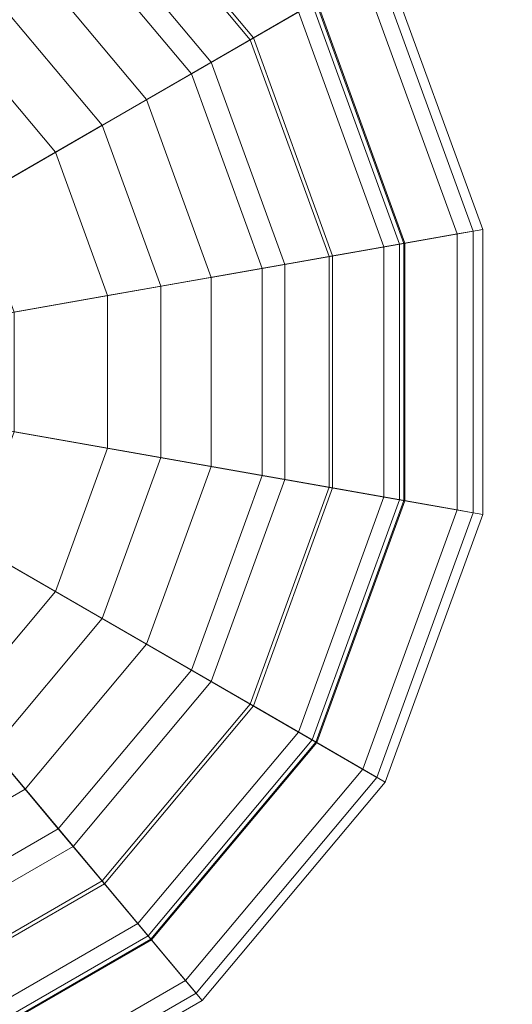
# Model space of a CAD drawing. Units: inches. Extents: x 375 to 1122, y 27 to 1069.
# Tile 130 of 155: x 722.65 to 723.463, y 901.45 to 903.075. Entities that reach past the tile are written whole.
import ezdxf

# ---------------------------------------------------------------- set-up
doc = ezdxf.new("R2010")
doc.units = ezdxf.units.IN
doc.layers.add('A-ANNO-DIMS', color=2, linetype='Continuous', lineweight=18)
doc.layers.add('Furniture', color=30, linetype='Continuous', lineweight=18)
doc.styles.get("Standard").update_dxf_attribs({"font": 'arial.ttf'})
doc.dimstyles.new('ISO-25', dxfattribs={"dimtxt": 12, "dimasz": 2.5, "dimexe": 1.5, "dimexo": 1.5, "dimtad": 1, "dimdec": 1, "dimlunit": 3, "dimtxsty": 'Standard', "dimblk": 'ARCHTICK', "dimcen": 2.5, "dimadec": 0, "dimazin": 0, "dimtfac": 1, "dimtdec": 1, "dimtmove": 0, "dimatfit": 3, "dimfxl": 1.5, "dimfxlon": 1, "dimarcsym": 0})

# ---------------------------------------------------------------- blocks, each defined once
blk = doc.blocks.new('A$C403C54AD')
for points in [[(0.890422, 0.958466, -0.039553), (0.889855, 0.961682, -0.042784), (0.878804, 0.95766, -0.042784), (0.880436, 0.954832, -0.039553)], [(0.889855, 0.961682, -0.042784), (0.895735, 0.928335, -0.039705), (0.895735, 0.928335, -0.039705), (0.878804, 0.95766, -0.042784)], [(0.901048, 0.958466, -0.039553), (0.901615, 0.961682, -0.042784), (0.889855, 0.961682, -0.042784), (0.890422, 0.958466, -0.039553)], [(0.901615, 0.961682, -0.042784), (0.895735, 0.928335, -0.039705), (0.895735, 0.928335, -0.039705), (0.889855, 0.961682, -0.042784)], [(0.912666, 0.95766, -0.042784), (0.895735, 0.928335, -0.039705), (0.895735, 0.928335, -0.039705), (0.901615, 0.961682, -0.042784)], [(0.911033, 0.954832, -0.039553), (0.912666, 0.95766, -0.042784), (0.901615, 0.961682, -0.042784), (0.901048, 0.958466, -0.039553)], [(0.890429, 0.958426, 0.1202), (0.889924, 0.961289, 0.106976), (0.879003, 0.957315, 0.106976), (0.880457, 0.954797, 0.1202)], [(0.889924, 0.961289, 0.106976), (0.890041, 0.960625, 0.078734), (0.87934, 0.95673, 0.078734), (0.879003, 0.957315, 0.106976)], [(0.901041, 0.958426, 0.1202), (0.901545, 0.961289, 0.106976), (0.889924, 0.961289, 0.106976), (0.890429, 0.958426, 0.1202)], [(0.901545, 0.961289, 0.106976), (0.901428, 0.960625, 0.078734), (0.890041, 0.960625, 0.078734), (0.889924, 0.961289, 0.106976)], [(0.911013, 0.954797, 0.1202), (0.912466, 0.957315, 0.106976), (0.901545, 0.961289, 0.106976), (0.901041, 0.958426, 0.1202)], [(0.912466, 0.957315, 0.106976), (0.912129, 0.95673, 0.078734), (0.901428, 0.960625, 0.078734), (0.901545, 0.961289, 0.106976)], [(0.890041, 0.960625, 0.078734), (0.890973, 0.955342, 0.060725), (0.882023, 0.952084, 0.060725), (0.87934, 0.95673, 0.078734)], [(0.901428, 0.960625, 0.078734), (0.900497, 0.955342, 0.060725), (0.890973, 0.955342, 0.060725), (0.890041, 0.960625, 0.078734)], [(0.912129, 0.95673, 0.078734), (0.909447, 0.952084, 0.060725), (0.900497, 0.955342, 0.060725), (0.901428, 0.960625, 0.078734)], [(0.893266, 0.942333, -0.036278), (0.890422, 0.958466, -0.039553), (0.880436, 0.954832, -0.039553), (0.888627, 0.940645, -0.036278)], [(0.891296, 0.953506, 0.129606), (0.890429, 0.958426, 0.1202), (0.880457, 0.954797, 0.1202), (0.882955, 0.95047, 0.129606)], [(0.890459, 0.958252, 0.106759), (0.890947, 0.955485, 0.119395), (0.88195, 0.95221, 0.119395), (0.880545, 0.954643, 0.106759)], [(0.890574, 0.957604, 0.079219), (0.890459, 0.958252, 0.106759), (0.880545, 0.954643, 0.106759), (0.880874, 0.954073, 0.079219)], [(0.898203, 0.942333, -0.036278), (0.901048, 0.958466, -0.039553), (0.890422, 0.958466, -0.039553), (0.893266, 0.942333, -0.036278)], [(0.900173, 0.953506, 0.129606), (0.901041, 0.958426, 0.1202), (0.890429, 0.958426, 0.1202), (0.891296, 0.953506, 0.129606)], [(0.90101, 0.958252, 0.106759), (0.900522, 0.955485, 0.119395), (0.890947, 0.955485, 0.119395), (0.890459, 0.958252, 0.106759)], [(0.900896, 0.957604, 0.079219), (0.90101, 0.958252, 0.106759), (0.890459, 0.958252, 0.106759), (0.890574, 0.957604, 0.079219)], [(0.902842, 0.940645, -0.036278), (0.911033, 0.954832, -0.039553), (0.901048, 0.958466, -0.039553), (0.898203, 0.942333, -0.036278)], [(0.908514, 0.95047, 0.129606), (0.911013, 0.954797, 0.1202), (0.901041, 0.958426, 0.1202), (0.900173, 0.953506, 0.129606)], [(0.910924, 0.954643, 0.106759), (0.909519, 0.95221, 0.119395), (0.900522, 0.955485, 0.119395), (0.90101, 0.958252, 0.106759)], [(0.910595, 0.954073, 0.079219), (0.910924, 0.954643, 0.106759), (0.90101, 0.958252, 0.106759), (0.900896, 0.957604, 0.079219)], [(0.878804, 0.95766, -0.042784), (0.895735, 0.928335, -0.039705), (0.895735, 0.928335, -0.039705), (0.869795, 0.950101, -0.042784)], [(0.891461, 0.952574, 0.062072), (0.890574, 0.957604, 0.079219), (0.880874, 0.954073, 0.079219), (0.883428, 0.94965, 0.062072)], [(0.900009, 0.952574, 0.062072), (0.900896, 0.957604, 0.079219), (0.890574, 0.957604, 0.079219), (0.891461, 0.952574, 0.062072)], [(0.921675, 0.950101, -0.042784), (0.895735, 0.928335, -0.039705), (0.895735, 0.928335, -0.039705), (0.912666, 0.95766, -0.042784)], [(0.908041, 0.94965, 0.062072), (0.910595, 0.954073, 0.079219), (0.900896, 0.957604, 0.079219), (0.900009, 0.952574, 0.062072)], [(0.919173, 0.948002, -0.039553), (0.921675, 0.950101, -0.042784), (0.912666, 0.95766, -0.042784), (0.911033, 0.954832, -0.039553)], [(0.919142, 0.947976, 0.1202), (0.921369, 0.949844, 0.106976), (0.912466, 0.957315, 0.106976), (0.911013, 0.954797, 0.1202)], [(0.921369, 0.949844, 0.106976), (0.920852, 0.949411, 0.078734), (0.912129, 0.95673, 0.078734), (0.912466, 0.957315, 0.106976)], [(0.87934, 0.95673, 0.078734), (0.882023, 0.952084, 0.060725), (0.874727, 0.945962, 0.060725), (0.870617, 0.949411, 0.078734)], [(0.920852, 0.949411, 0.078734), (0.916743, 0.945962, 0.060725), (0.909447, 0.952084, 0.060725), (0.912129, 0.95673, 0.078734)], [(0.890947, 0.955485, 0.119395), (0.891831, 0.950474, 0.129606), (0.884494, 0.947804, 0.129606), (0.88195, 0.95221, 0.119395)], [(0.890973, 0.955342, 0.060725), (0.8922, 0.948383, 0.050493), (0.885556, 0.945965, 0.050493), (0.882023, 0.952084, 0.060725)], [(0.900522, 0.955485, 0.119395), (0.899638, 0.950474, 0.129606), (0.891831, 0.950474, 0.129606), (0.890947, 0.955485, 0.119395)], [(0.900497, 0.955342, 0.060725), (0.89927, 0.948383, 0.050493), (0.8922, 0.948383, 0.050493), (0.890973, 0.955342, 0.060725)], [(0.909447, 0.952084, 0.060725), (0.905913, 0.945965, 0.050493), (0.89927, 0.948383, 0.050493), (0.900497, 0.955342, 0.060725)], [(0.909519, 0.95221, 0.119395), (0.906975, 0.947804, 0.129606), (0.899638, 0.950474, 0.129606), (0.900522, 0.955485, 0.119395)], [(0.888627, 0.940645, -0.036278), (0.880436, 0.954832, -0.039553), (0.872296, 0.948002, -0.039553), (0.884846, 0.937471, -0.036278)], [(0.882955, 0.95047, 0.129606), (0.880457, 0.954797, 0.1202), (0.872327, 0.947976, 0.1202), (0.876155, 0.944764, 0.129606)], [(0.880545, 0.954643, 0.106759), (0.88195, 0.95221, 0.119395), (0.874615, 0.946056, 0.119395), (0.872463, 0.947862, 0.106759)], [(0.906623, 0.937471, -0.036278), (0.919173, 0.948002, -0.039553), (0.911033, 0.954832, -0.039553), (0.902842, 0.940645, -0.036278)], [(0.915314, 0.944764, 0.129606), (0.919142, 0.947976, 0.1202), (0.911013, 0.954797, 0.1202), (0.908514, 0.95047, 0.129606)], [(0.919006, 0.947862, 0.106759), (0.916854, 0.946056, 0.119395), (0.909519, 0.95221, 0.119395), (0.910924, 0.954643, 0.106759)], [(0.918502, 0.947439, 0.079219), (0.919006, 0.947862, 0.106759), (0.910924, 0.954643, 0.106759), (0.910595, 0.954073, 0.079219)], [(0.883428, 0.94965, 0.062072), (0.880874, 0.954073, 0.079219), (0.872967, 0.947439, 0.079219), (0.87688, 0.944156, 0.062072)], [(0.914589, 0.944156, 0.062072), (0.918502, 0.947439, 0.079219), (0.910595, 0.954073, 0.079219), (0.908041, 0.94965, 0.062072)], [(0.891831, 0.950474, 0.129606), (0.891296, 0.953506, 0.129606), (0.882955, 0.95047, 0.129606), (0.884494, 0.947804, 0.129606)], [(0.899638, 0.950474, 0.129606), (0.900173, 0.953506, 0.129606), (0.891296, 0.953506, 0.129606), (0.891831, 0.950474, 0.129606)], [(0.906975, 0.947804, 0.129606), (0.908514, 0.95047, 0.129606), (0.900173, 0.953506, 0.129606), (0.899638, 0.950474, 0.129606)], [(0.892587, 0.946186, 0.05268), (0.891461, 0.952574, 0.062072), (0.883428, 0.94965, 0.062072), (0.886671, 0.944033, 0.05268)], [(0.898882, 0.946186, 0.05268), (0.900009, 0.952574, 0.062072), (0.891461, 0.952574, 0.062072), (0.892587, 0.946186, 0.05268)], [(0.904798, 0.944033, 0.05268), (0.908041, 0.94965, 0.062072), (0.900009, 0.952574, 0.062072), (0.898882, 0.946186, 0.05268)], [(0.88195, 0.95221, 0.119395), (0.884494, 0.947804, 0.129606), (0.878513, 0.942785, 0.129606), (0.874615, 0.946056, 0.119395)], [(0.882023, 0.952084, 0.060725), (0.885556, 0.945965, 0.050493), (0.88014, 0.94142, 0.050493), (0.874727, 0.945962, 0.060725)], [(0.916743, 0.945962, 0.060725), (0.911329, 0.94142, 0.050493), (0.905913, 0.945965, 0.050493), (0.909447, 0.952084, 0.060725)], [(0.916854, 0.946056, 0.119395), (0.912956, 0.942785, 0.129606), (0.906975, 0.947804, 0.129606), (0.909519, 0.95221, 0.119395)], [(0.884494, 0.947804, 0.129606), (0.882955, 0.95047, 0.129606), (0.876155, 0.944764, 0.129606), (0.878513, 0.942785, 0.129606)], [(0.912956, 0.942785, 0.129606), (0.915314, 0.944764, 0.129606), (0.908514, 0.95047, 0.129606), (0.906975, 0.947804, 0.129606)], [(0.869795, 0.950101, -0.042784), (0.895735, 0.928335, -0.039705), (0.895735, 0.928335, -0.039705), (0.863915, 0.939916, -0.042784)], [(0.927555, 0.939916, -0.042784), (0.895735, 0.928335, -0.039705), (0.895735, 0.928335, -0.039705), (0.921675, 0.950101, -0.042784)], [(0.924486, 0.938799, -0.039553), (0.927555, 0.939916, -0.042784), (0.921675, 0.950101, -0.042784), (0.919173, 0.948002, -0.039553)], [(0.886671, 0.944033, 0.05268), (0.883428, 0.94965, 0.062072), (0.87688, 0.944156, 0.062072), (0.881848, 0.939987, 0.05268)], [(0.909621, 0.939987, 0.05268), (0.914589, 0.944156, 0.062072), (0.908041, 0.94965, 0.062072), (0.904798, 0.944033, 0.05268)], [(0.924448, 0.938785, 0.1202), (0.92718, 0.93978, 0.106976), (0.921369, 0.949844, 0.106976), (0.919142, 0.947976, 0.1202)], [(0.92718, 0.93978, 0.106976), (0.926546, 0.939549, 0.078734), (0.920852, 0.949411, 0.078734), (0.921369, 0.949844, 0.106976)], [(0.926546, 0.939549, 0.078734), (0.921505, 0.937714, 0.060725), (0.916743, 0.945962, 0.060725), (0.920852, 0.949411, 0.078734)], [(0.884846, 0.937471, -0.036278), (0.872296, 0.948002, -0.039553), (0.866983, 0.938799, -0.039553), (0.882378, 0.933196, -0.036278)], [(0.8922, 0.948383, 0.050493), (0.893978, 0.9383, 0.043125), (0.890675, 0.937098, 0.043125), (0.885556, 0.945965, 0.050493)], [(0.89927, 0.948383, 0.050493), (0.897492, 0.9383, 0.043125), (0.893978, 0.9383, 0.043125), (0.8922, 0.948383, 0.050493)], [(0.905913, 0.945965, 0.050493), (0.900794, 0.937098, 0.043125), (0.897492, 0.9383, 0.043125), (0.89927, 0.948383, 0.050493)], [(0.909092, 0.933196, -0.036278), (0.924486, 0.938799, -0.039553), (0.919173, 0.948002, -0.039553), (0.906623, 0.937471, -0.036278)], [(0.919753, 0.937076, 0.129606), (0.924448, 0.938785, 0.1202), (0.919142, 0.947976, 0.1202), (0.915314, 0.944764, 0.129606)], [(0.924281, 0.938725, 0.106759), (0.921641, 0.937764, 0.119395), (0.916854, 0.946056, 0.119395), (0.919006, 0.947862, 0.106759)], [(0.923663, 0.9385, 0.079219), (0.924281, 0.938725, 0.106759), (0.919006, 0.947862, 0.106759), (0.918502, 0.947439, 0.079219)], [(0.918863, 0.936753, 0.062072), (0.923663, 0.9385, 0.079219), (0.918502, 0.947439, 0.079219), (0.914589, 0.944156, 0.062072)], [(0.894188, 0.937103, 0.046044), (0.892587, 0.946186, 0.05268), (0.886671, 0.944033, 0.05268), (0.891283, 0.936046, 0.046044)], [(0.897281, 0.937103, 0.046044), (0.898882, 0.946186, 0.05268), (0.892587, 0.946186, 0.05268), (0.894188, 0.937103, 0.046044)], [(0.900187, 0.936046, 0.046044), (0.904798, 0.944033, 0.05268), (0.898882, 0.946186, 0.05268), (0.897281, 0.937103, 0.046044)], [(0.921641, 0.937764, 0.119395), (0.91686, 0.936024, 0.129606), (0.912956, 0.942785, 0.129606), (0.916854, 0.946056, 0.119395)], [(0.885556, 0.945965, 0.050493), (0.890675, 0.937098, 0.043125), (0.887983, 0.934839, 0.043125), (0.88014, 0.94142, 0.050493)], [(0.911329, 0.94142, 0.050493), (0.903486, 0.934839, 0.043125), (0.900794, 0.937098, 0.043125), (0.905913, 0.945965, 0.050493)], [(0.921505, 0.937714, 0.060725), (0.914864, 0.935297, 0.050493), (0.911329, 0.94142, 0.050493), (0.916743, 0.945962, 0.060725)], [(0.91686, 0.936024, 0.129606), (0.919753, 0.937076, 0.129606), (0.915314, 0.944764, 0.129606), (0.912956, 0.942785, 0.129606)], [(0.881848, 0.939987, 0.05268), (0.87688, 0.944156, 0.062072), (0.872606, 0.936753, 0.062072), (0.878701, 0.934534, 0.05268)], [(0.891283, 0.936046, 0.046044), (0.886671, 0.944033, 0.05268), (0.881848, 0.939987, 0.05268), (0.888914, 0.934058, 0.046044)], [(0.902556, 0.934058, 0.046044), (0.909621, 0.939987, 0.05268), (0.904798, 0.944033, 0.05268), (0.900187, 0.936046, 0.046044)], [(0.912769, 0.934534, 0.05268), (0.918863, 0.936753, 0.062072), (0.914589, 0.944156, 0.062072), (0.909621, 0.939987, 0.05268)]]:
    blk.add_3dface(points)
blk = doc.blocks.new('_ArchTick')
at = {"color": 0, "linetype": 'ByBlock', "const_width": 0.15}
blk.add_lwpolyline([(-0.5, -0.5), (0.5, 0.5)], dxfattribs=at)
blk = doc.blocks.new('*D73')
at = {"layer": 'A-ANNO-DIMS', "color": 0, "lineweight": -2, "transparency": 16777216}
for p, q in [((686.7573, 932.4277), (686.7573, 929.4277)), ((770.7573, 932.4277), (770.7573, 929.4277)), ((686.7573, 930.9277), (770.7573, 930.9277)), ((770.7573, 930.9277), (987.6096, 930.9277))]:
    blk.add_line(p, q, dxfattribs=at)
at = {"layer": 'Defpoints', "color": 0, "transparency": 16777216}
for p in [(686.7573, 943.5277), (770.7573, 943.5277), (770.7573, 930.9277)]:
    blk.add_point(p, dxfattribs=at)
at = {"layer": 'A-ANNO-DIMS', "color": 0, "lineweight": -2, "transparency": 16777216, "xscale": 2.5, "yscale": 2.5, "zscale": 2.5, "rotation": 180}
blk.add_blockref('_ArchTick', (686.7573, 930.9277), dxfattribs=at)
at = {"layer": 'A-ANNO-DIMS', "color": 0, "lineweight": -2, "transparency": 16777216, "xscale": 2.5, "yscale": 2.5, "zscale": 2.5}
blk.add_blockref('_ArchTick', (770.7573, 930.9277), dxfattribs=at)
at = {"layer": 'A-ANNO-DIMS', "color": 0, "transparency": 16777216, "insert": (880.4335, 937.7573), "char_height": 12, "attachment_point": 5}
blk.add_mtext('2-PANEL SLIDER 7\'-0" TYP.', dxfattribs=at)

msp = doc.modelspace()

# ---------------------------------------------------------------- block references
at = {"layer": 'Furniture', "xscale": 39.9918517141215, "yscale": 39.9918517141215, "zscale": 39.9918517141215, "rotation": 270}
msp.add_blockref('A$C403C54AD', (684.9549, 938.3156, 0.024), dxfattribs=at)

# ---------------------------------------------------------------- dimensions: what is measured, and where the dimension line sits
at = {"layer": 'A-ANNO-DIMS'}
dim = msp.add_linear_dim(base=(770.7573, 930.9277), p1=(686.7573, 943.5277), p2=(770.7573, 943.5277), text='2-PANEL SLIDER <> TYP.', dimstyle='ISO-25', override={"dimdec": 1, "dimlfac": 1, "dimrnd": 0, "dimzin": 1, "dimdsep": 46, "dimlunit": 4, "dimfrac": 2}, dxfattribs=at)
dim.commit()
dim.dimension.update_dxf_attribs({"geometry": '*D73', "text_midpoint": (880.4335, 937.7573)})

doc.saveas('drawing.dxf')
